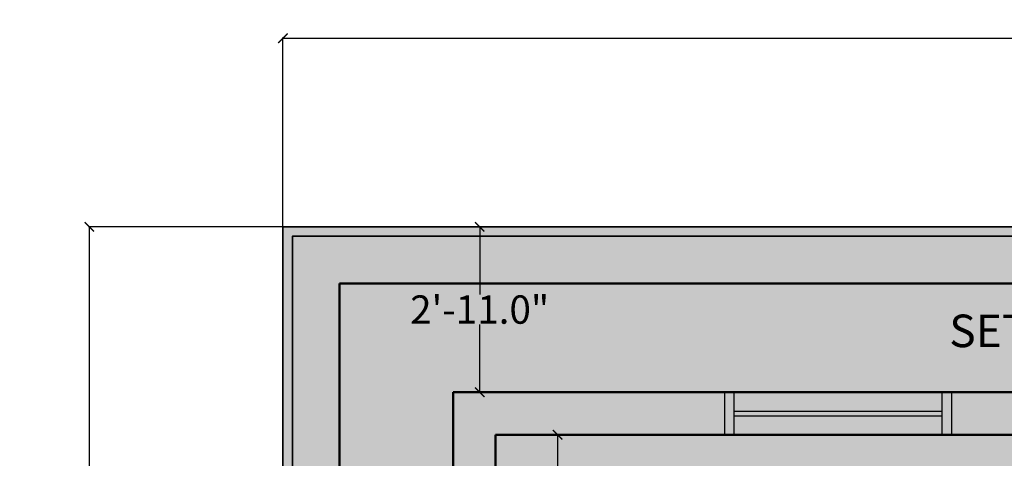
# Model space of a CAD drawing. Units: inches. Extents: x 528 to 2620, y -1066 to 798.
# Tile 9 of 41: x 528 to 737, y 705 to 798. Entities that reach past the tile are written whole.
import ezdxf

# ---------------------------------------------------------------- set-up
doc = ezdxf.new("R2010")
doc.units = ezdxf.units.IN
doc.header["$MEASUREMENT"] = 0
for name, color, linetype, lineweight in [('A-ANNO-DIMS', 2, 'Continuous', 18), ('A-AREA-IDEN', 7, 'Continuous', 18), ('A-GLAZ', 3, 'Continuous', 25), ('A-WALL', 7, 'Continuous', 50), ('A-WALL-PATT', 8, 'Continuous', 13), ('C-PROP', 5, 'Continuous', 35)]:
    doc.layers.add(name, color=color, linetype=linetype, lineweight=lineweight)
doc.styles.get("Standard").update_dxf_attribs({"font": 'arial.ttf'})
doc.dimstyles.get("Standard").update_dxf_attribs({"dimtxt": 6, "dimasz": 2, "dimexe": 0.18, "dimexo": 0.0625, "dimgap": 0.09, "dimtad": 0, "dimtih": 1, "dimtoh": 1, "dimdec": 1, "dimzin": 0, "dimdsep": 46, "dimlunit": 3, "dimtxsty": 'Standard', "dimblk": 'ARCHTICK', "dimcen": 0.09, "dimadec": 0, "dimazin": 0, "dimtfac": 1, "dimtdec": 1, "dimtofl": 0, "dimtmove": 0, "dimatfit": 3, "dimfxl": 1, "dimtolj": 1, "dimtzin": 0, "dimarcsym": 0})

# ---------------------------------------------------------------- blocks, each defined once
blk = doc.blocks.new('_ArchTick')
at = {"color": 0, "linetype": 'ByBlock', "const_width": 0.15}
blk.add_lwpolyline([(-0.5, -0.5), (0.5, 0.5)], dxfattribs=at)
blk = doc.blocks.new('*D11')
at = {"layer": 'A-ANNO-DIMS', "color": 0, "lineweight": -2, "transparency": 16777216}
for p, q in [((584.06, 753.98), (584.06, 794.01)), ((584.06, 793.83), (758.88, 793.83)), ((944.06, 793.83), (769.24, 793.83)), ((944.06, 753.98), (944.06, 794.01))]:
    blk.add_line(p, q, dxfattribs=at)
at = {"layer": 'Defpoints', "color": 0, "transparency": 16777216}
for p in [(944.06, 793.83), (584.06, 753.92), (944.06, 753.92)]:
    blk.add_point(p, dxfattribs=at)
at = {"layer": 'A-ANNO-DIMS', "color": 0, "lineweight": -2, "transparency": 16777216, "xscale": 2, "yscale": 2, "zscale": 2, "rotation": 180}
blk.add_blockref('_ArchTick', (584.06, 793.83), dxfattribs=at)
at = {"layer": 'A-ANNO-DIMS', "color": 0, "lineweight": -2, "transparency": 16777216, "xscale": 2, "yscale": 2, "zscale": 2}
blk.add_blockref('_ArchTick', (944.06, 793.83), dxfattribs=at)
at = {"layer": 'A-ANNO-DIMS', "color": 0, "transparency": 16777216, "insert": (764.06, 793.83), "char_height": 6, "attachment_point": 5}
blk.add_mtext("\\A1;30'", dxfattribs=at)
blk = doc.blocks.new('*D12')
at = {"layer": 'A-ANNO-DIMS', "color": 0, "lineweight": -2, "transparency": 16777216}
for p, q in [((584, 753.92), (542.88, 753.92)), ((543.06, 753.92), (543.06, 484.58)), ((543.06, 208.92), (543.06, 478.27)), ((584, 208.92), (542.88, 208.92))]:
    blk.add_line(p, q, dxfattribs=at)
at = {"layer": 'Defpoints', "color": 0, "transparency": 16777216}
for p in [(584.06, 753.92), (543.06, 208.92), (584.06, 208.92)]:
    blk.add_point(p, dxfattribs=at)
at = {"layer": 'A-ANNO-DIMS', "color": 0, "lineweight": -2, "transparency": 16777216, "xscale": 2, "yscale": 2, "zscale": 2}
for p, rotation in [((543.06, 753.92), 90), ((543.06, 208.92), 270)]:
    blk.add_blockref('_ArchTick', p, dxfattribs=dict(at, rotation=rotation))
at = {"layer": 'A-ANNO-DIMS', "color": 0, "transparency": 16777216, "insert": (543.06, 481.42), "char_height": 6, "attachment_point": 5}
blk.add_mtext('\\A1;45\'-5.0"', dxfattribs=at)
blk = doc.blocks.new('*D13')
at = {"layer": 'A-ANNO-DIMS', "color": 0, "lineweight": -2, "transparency": 16777216}
for p, q in [((625.99, 753.92), (625.52, 753.92)), ((625.7, 753.92), (625.7, 739.58)), ((625.7, 718.92), (625.7, 733.27)), ((625.99, 718.92), (625.52, 718.92))]:
    blk.add_line(p, q, dxfattribs=at)
at = {"layer": 'Defpoints', "color": 0, "transparency": 16777216}
for p in [(625.7, 753.92), (626.05, 753.92), (626.05, 718.92)]:
    blk.add_point(p, dxfattribs=at)
at = {"layer": 'A-ANNO-DIMS', "color": 0, "lineweight": -2, "transparency": 16777216, "xscale": 2, "yscale": 2, "zscale": 2}
for p, rotation in [((625.7, 753.92), 90), ((625.7, 718.92), 270)]:
    blk.add_blockref('_ArchTick', p, dxfattribs=dict(at, rotation=rotation))
at = {"layer": 'A-ANNO-DIMS', "color": 0, "transparency": 16777216, "insert": (625.7, 736.42), "char_height": 6, "attachment_point": 5}
blk.add_mtext('\\A1;2\'-11.0"', dxfattribs=at)
blk = doc.blocks.new('*D26')
at = {"layer": 'A-ANNO-DIMS', "color": 0, "lineweight": -2, "transparency": 16777216}
for p, q in [((642.51, 709.92), (641.99, 709.92)), ((642.17, 709.92), (642.17, 647.02)), ((642.17, 577.92), (642.17, 640.82)), ((642.51, 577.92), (641.99, 577.92))]:
    blk.add_line(p, q, dxfattribs=at)
at = {"layer": 'Defpoints', "color": 0, "transparency": 16777216}
for p in [(642.57, 709.92), (642.17, 577.92), (642.57, 577.92)]:
    blk.add_point(p, dxfattribs=at)
at = {"layer": 'A-ANNO-DIMS', "color": 0, "lineweight": -2, "transparency": 16777216, "xscale": 2, "yscale": 2, "zscale": 2}
for p, rotation in [((642.17, 709.92), 90), ((642.17, 577.92), 270)]:
    blk.add_blockref('_ArchTick', p, dxfattribs=dict(at, rotation=rotation))
at = {"layer": 'A-ANNO-DIMS', "color": 0, "transparency": 16777216, "insert": (642.17, 643.92), "char_height": 6, "attachment_point": 5}
blk.add_mtext("\\A1;11'", dxfattribs=at)
blk = doc.blocks.new('WIN-1200')
for p, q in [((677.56, 718.92), (725.56, 718.92)), ((677.56, 709.92), (677.56, 718.92)), ((679.56, 709.92), (679.56, 718.92)), ((723.56, 718.92), (723.56, 709.92)), ((725.56, 718.92), (725.56, 709.92)), ((679.56, 714.92), (723.56, 714.92)), ((679.56, 713.92), (723.56, 713.92)), ((725.56, 709.92), (677.56, 709.92))]:
    blk.add_line(p, q)

msp = doc.modelspace()

# ---------------------------------------------------------------- hatches: boundary and pattern name
at = {"layer": 'A-WALL-PATT', "transparency": 33554687}
h = msp.add_hatch(color=256, dxfattribs=at)
h.dxf.hatch_style = 1
h.paths.add_polyline_path([(944.06, 753.92), (584.06, 753.92), (584.06, 208.92), (608.06, 208.92), (608.06, 210.92), (586.06, 210.92), (586.06, 751.92), (942.06, 751.92), (942.06, 210.92), (728.06, 210.92), (728.06, 208.92), (944.06, 208.92)])
h = msp.add_hatch(color=256, dxfattribs=at)
h.dxf.hatch_style = 1
h.paths.add_polyline_path([(942.06, 751.92), (586.06, 751.92), (586.06, 210.92), (608.06, 210.92), (608.06, 220.92), (596.06, 220.92), (596.06, 741.92), (932.06, 741.92), (932.06, 220.92), (770.06, 220.92), (728.06, 220.92), (728.06, 210.92), (942.06, 210.92)])
at = {"layer": 'A-WALL-PATT', "transparency": 33554475}
h = msp.add_hatch(color=256, dxfattribs=at)
h.dxf.hatch_style = 1
h.paths.add_polyline_path([(620.06, 718.92), (908.06, 718.92), (908.06, 268.92), (770.06, 268.92), (770.06, 220.92), (932.06, 220.92), (932.06, 741.92), (596.06, 741.92), (596.06, 391.42), (620.06, 391.42)])
at = {"layer": 'A-WALL-PATT', "transparency": 33554687}
h = msp.add_hatch(color=256, dxfattribs=at)
h.dxf.hatch_style = 1
h.paths.add_polyline_path([(861.06, 273.92), (817.06, 273.92), (817.06, 272.92), (861.06, 272.92)])
h.paths.add_polyline_path([(817.06, 277.92), (815.06, 277.92), (815.06, 268.92), (817.06, 268.92)])
h.paths.add_polyline_path([(908.06, 397.92), (899.06, 397.92), (899.06, 395.92), (908.06, 395.92)])
h.paths.add_polyline_path([(908.06, 443.92), (899.06, 443.92), (899.06, 441.92), (908.06, 441.92)])
h.paths.add_polyline_path([(904.06, 441.92), (903.06, 441.92), (903.06, 397.92), (904.06, 397.92)])
h.paths.add_polyline_path([(625.06, 561.42), (624.06, 561.42), (624.06, 537.42), (625.06, 537.42)])
h.paths.add_polyline_path([(648.75, 334.44), (720.04, 334.44), (720.04, 345), (648.75, 345)], flags=9)
h.paths.add_polyline_path([(819.73, 323.15), (880.33, 323.15), (880.33, 333.71), (819.73, 333.71)], flags=9)
h.paths.add_polyline_path([(779.9, 680.61), (821.76, 680.61), (821.76, 691.17), (779.9, 691.17)], flags=9)
h.paths.add_polyline_path([(779.88, 692.36), (817.14, 692.36), (817.14, 703.06), (779.88, 703.06)], flags=9)
h.paths.add_polyline_path([(799.99, 453.88), (860.59, 453.88), (860.59, 464.44), (799.99, 464.44)], flags=9)
h.paths.add_polyline_path([(650.87, 539.4), (708.78, 539.4), (708.78, 549.95), (650.87, 549.95)], flags=9)
h.paths.add_polyline_path([(788.5, 612.01), (849.1, 612.01), (849.1, 622.56), (788.5, 622.56)], flags=9)
h.paths.add_polyline_path([(639.54, 648.31), (700.13, 648.31), (700.13, 658.87), (639.54, 658.87)], flags=9)
h.paths.add_polyline_path([(648.91, 346.09), (747.71, 346.09), (747.71, 356.78), (648.91, 356.78)], flags=9)
h.paths.add_polyline_path([(676.86, 450.66), (746.74, 450.66), (746.74, 461.36), (676.86, 461.36)], flags=9)
h.paths.add_polyline_path([(819.71, 334.95), (865.53, 334.95), (865.53, 345.64), (819.71, 345.64)], flags=9)
h.paths.add_polyline_path([(806.3, 467.75), (874.05, 467.75), (874.05, 478.44), (806.3, 478.44)], flags=9)
h.paths.add_polyline_path([(653.23, 552.28), (690.5, 552.28), (690.5, 562.98), (653.23, 562.98)], flags=9)
h.paths.add_polyline_path([(789.9, 623.41), (843.21, 623.41), (843.21, 634.1), (789.9, 634.1)], flags=9)
h.paths.add_polyline_path([(639.77, 662.1), (693.08, 662.1), (693.08, 672.8), (639.77, 672.8)], flags=9)
h.paths.add_polyline_path([(801.59, 242.91), (846.33, 242.91), (846.33, 253.6), (801.59, 253.6)], flags=9)
h.paths.add_polyline_path([(925.36, 593.98), (925.36, 674.06), (914.67, 674.06), (914.67, 593.98)], flags=9)
h.paths.add_polyline_path([(612.56, 593.98), (612.56, 674.06), (601.87, 674.06), (601.87, 593.98)], flags=9)
h.paths.add_polyline_path([(723.31, 726.56), (803.39, 726.56), (803.39, 737.25), (723.31, 737.25)], flags=9)
at = {"layer": 'A-WALL-PATT', "transparency": 33554521}
h = msp.add_hatch(color=256, dxfattribs=at)
h.dxf.hatch_style = 1
h.paths.add_polyline_path([(629.06, 709.92), (677.56, 709.92), (677.56, 718.92), (620.06, 718.92), (620.06, 667.92), (629.06, 667.92)])
h.paths.add_polyline_path([(790.56, 718.92), (725.56, 718.92), (725.56, 709.92), (774.06, 709.92), (774.06, 577.92), (768.48, 577.92), (768.56, 573.42), (774.06, 573.42), (774.06, 567.42), (778.56, 567.42), (778.56, 669.42), (831.06, 669.42), (831.06, 675.92), (826.56, 675.92), (826.56, 673.92), (778.56, 673.92), (778.56, 709.92), (790.56, 709.92)])
h.paths.add_polyline_path([(908.06, 718.92), (879.06, 718.92), (879.06, 709.92), (899.06, 709.92), (899.06, 641.67), (908.06, 641.67)])
h.paths.add_polyline_path([(629.06, 619.92), (620.06, 619.92), (620.06, 561.42), (629.06, 561.42), (629.06, 573.42), (724.06, 573.42), (724.06, 569.42), (728.56, 569.42), (728.56, 577.92), (629.06, 577.92)])
h.paths.add_polyline_path([(779.06, 391.42), (779.06, 400.42), (770.06, 400.42), (764.06, 400.42), (764.06, 397.42), (764.06, 391.42), (770.06, 391.42), (770.06, 268.92), (815.06, 268.92), (815.06, 277.92), (779.06, 277.92), (779.06, 359.77)])
h.paths.add_polyline_path([(908.06, 395.92), (899.06, 395.92), (851.06, 395.92), (851.06, 391.42), (899.06, 391.42), (899.06, 277.92), (863.06, 277.92), (863.06, 268.92), (908.06, 268.92)])
h.paths.add_polyline_path([(908.06, 593.67), (899.06, 593.67), (899.06, 525.42), (778.56, 525.42), (778.56, 527.17), (774.06, 527.17), (774.06, 520.92), (899.06, 520.92), (899.06, 443.92), (908.06, 443.92)])
h.paths.add_polyline_path([(629.06, 520.92), (728.56, 520.92), (728.56, 545.42), (724.06, 545.42), (724.06, 525.42), (629.06, 525.42), (629.06, 537.42), (620.06, 537.42), (620.06, 484.67), (629.06, 484.67)])
h.paths.add_polyline_path([(629.06, 436.67), (620.06, 436.67), (620.06, 391.42), (648.56, 391.42), (648.56, 400.42), (629.06, 400.42)])
h.paths.add_polyline_path([(716.06, 397.42), (716.06, 400.42), (696.56, 400.42), (696.56, 391.42), (716.06, 391.42)])
at = {"layer": 'A-WALL-PATT', "transparency": 33554681}
h = msp.add_hatch(color=256, dxfattribs=at)
h.dxf.hatch_style = 1
h.paths.add_polyline_path([(629.06, 665.92), (625.06, 665.92), (625.06, 621.92), (629.06, 621.92)])
h.paths.add_polyline_path([(624.06, 665.92), (620.06, 665.92), (620.06, 621.92), (624.06, 621.92)])
h.paths.add_polyline_path([(723.56, 713.92), (679.56, 713.92), (679.56, 709.92), (723.56, 709.92)])
h.paths.add_polyline_path([(723.56, 718.92), (679.56, 718.92), (679.56, 714.92), (723.56, 714.92)])
h.paths.add_polyline_path([(814.56, 713.92), (790.56, 713.92), (790.56, 709.92), (814.56, 709.92)])
h.paths.add_polyline_path([(814.56, 718.92), (790.56, 718.92), (790.56, 714.92), (814.56, 714.92)])
h.paths.add_polyline_path([(877.06, 713.92), (833.06, 713.92), (833.06, 709.92), (877.06, 709.92)])
h.paths.add_polyline_path([(877.06, 718.92), (833.06, 718.92), (833.06, 714.92), (877.06, 714.92)])
h.paths.add_polyline_path([(908.06, 639.67), (904.06, 639.67), (904.06, 595.67), (908.06, 595.67)])
h.paths.add_polyline_path([(903.06, 639.67), (899.06, 639.67), (899.06, 595.67), (903.06, 595.67)])
h.paths.add_polyline_path([(908.06, 441.92), (904.06, 441.92), (904.06, 397.92), (908.06, 397.92)])
h.paths.add_polyline_path([(903.06, 441.92), (899.06, 441.92), (899.06, 397.92), (903.06, 397.92)])
h.paths.add_polyline_path([(861.06, 272.92), (817.06, 272.92), (817.06, 268.92), (861.06, 268.92)])
h.paths.add_polyline_path([(861.06, 277.92), (817.06, 277.92), (817.06, 273.92), (861.06, 273.92)])
h.paths.add_polyline_path([(694.56, 395.42), (650.56, 395.42), (650.56, 391.42), (694.56, 391.42)])
h.paths.add_polyline_path([(694.56, 400.42), (650.56, 400.42), (650.56, 396.42), (694.56, 396.42)])
h.paths.add_polyline_path([(629.06, 482.67), (625.06, 482.67), (625.06, 438.67), (629.06, 438.67)])
h.paths.add_polyline_path([(624.06, 482.67), (620.06, 482.67), (620.06, 438.67), (624.06, 438.67)])
h.paths.add_polyline_path([(629.06, 561.42), (625.06, 561.42), (625.06, 537.42), (629.06, 537.42)])
h.paths.add_polyline_path([(624.06, 561.42), (620.06, 561.42), (620.06, 537.42), (624.06, 537.42)])
h = msp.add_hatch(color=256, dxfattribs=at)
h.dxf.hatch_style = 1
h.paths.add_polyline_path([(625.06, 665.92), (624.06, 665.92), (624.06, 621.92), (625.06, 621.92)])
h.paths.add_polyline_path([(629.06, 667.92), (620.06, 667.92), (620.06, 665.92), (629.06, 665.92)])
h.paths.add_polyline_path([(629.06, 621.92), (620.06, 621.92), (620.06, 619.92), (629.06, 619.92)])
h.paths.add_polyline_path([(723.56, 714.92), (679.56, 714.92), (679.56, 713.92), (723.56, 713.92)])
h.paths.add_polyline_path([(725.56, 718.92), (723.56, 718.92), (723.56, 709.92), (725.56, 709.92)])
h.paths.add_polyline_path([(679.56, 718.92), (677.56, 718.92), (677.56, 709.92), (679.56, 709.92)])
h.paths.add_polyline_path([(814.56, 714.92), (790.56, 714.92), (790.56, 713.92), (814.56, 713.92)])
h.paths.add_polyline_path([(877.06, 714.92), (833.06, 714.92), (833.06, 713.92), (877.06, 713.92)])
h.paths.add_polyline_path([(879.06, 718.92), (877.06, 718.92), (877.06, 709.92), (879.06, 709.92)])
h.paths.add_polyline_path([(833.06, 718.92), (831.06, 718.92), (831.06, 709.92), (833.06, 709.92)])
h.paths.add_polyline_path([(650.56, 400.42), (648.56, 400.42), (648.56, 391.42), (650.56, 391.42)])
h.paths.add_polyline_path([(694.56, 396.42), (650.56, 396.42), (650.56, 395.42), (694.56, 395.42)])
h.paths.add_polyline_path([(696.56, 400.42), (694.56, 400.42), (694.56, 391.42), (696.56, 391.42)])
h.paths.add_polyline_path([(629.06, 438.67), (620.06, 438.67), (620.06, 436.67), (629.06, 436.67)])
h.paths.add_polyline_path([(629.06, 484.67), (620.06, 484.67), (620.06, 482.67), (629.06, 482.67)])
h.paths.add_polyline_path([(625.06, 482.67), (624.06, 482.67), (624.06, 438.67), (625.06, 438.67)])
at = {"layer": 'A-WALL-PATT', "transparency": 33554590}
h = msp.add_hatch(color=256, dxfattribs=at)
h.dxf.hatch_style = 1
h.paths.add_polyline_path([(774.06, 709.92), (629.06, 709.92), (629.06, 577.92), (728.56, 577.92), (728.56, 579.42), (728.56, 619.42), (730.31, 619.42), (730.31, 619.38, -0.401453), (768.56, 579.42), (768.56, 577.92), (774.06, 577.92)])
h.paths.add_polyline_path([(723.9, 686.06), (723.97, 686.06), (723.83, 686.13)], flags=0)
h.paths.add_polyline_path([(722.79, 642.7), (722.89, 642.76), (722.89, 684.99), (722.65, 685.24), (722.65, 685.82), (723.08, 686.26), (723.53, 686.26), (723.97, 686.06), (724.74, 686.13), (770.7, 686.13), (770.78, 686.14), (771.13, 686.27), (771.69, 686.09), (771.94, 685.48), (771.67, 684.9), (771.58, 684.87), (771.58, 642.78), (771.88, 642.51), (771.88, 641.92), (771.51, 641.46), (770.85, 641.46), (770.4, 641.83), (770.4, 641.55), (724.74, 641.55), (723.99, 641.7), (723.44, 641.41), (722.88, 641.59), (722.6, 642.14)], flags=16)
h.paths.add_polyline_path([(723.99, 641.7), (723.99, 641.71), (723.99, 641.7)], flags=0)
h.paths.add_polyline_path([(722.89, 642.73), (722.89, 684.99), (722.65, 685.24), (722.65, 685.82), (723.08, 686.26), (723.29, 686.26), (722.99, 686.17), (722.79, 685.97), (722.65, 685.68), (722.65, 685.43), (722.75, 685.14), (722.94, 684.94), (723.24, 684.81), (723.48, 684.81), (723.78, 684.9), (723.98, 685.1), (724.17, 685.49), (724.12, 685.64), (724.12, 685.25), (723.63, 684.75), (723.63, 642.96), (724.12, 642.51), (724.12, 641.89), (723.66, 641.46), (723.08, 641.46), (722.65, 641.9), (722.65, 642.48)], flags=0)
h.paths.add_polyline_path([(722.65, 642.29), (722.65, 642.04), (722.79, 641.75), (723.08, 641.46), (723.29, 641.46), (722.88, 641.59), (722.6, 642.14)], flags=0)
h.paths.add_polyline_path([(770.75, 686.13), (770.58, 686.13), (770.55, 686.06)], flags=0)
h.paths.add_polyline_path([(743.3, 645.29), (753.23, 659.4), (748.69, 663.75), (753.23, 668.54), (743.3, 682.46), (743.79, 682.59), (744.14, 682.68), (744.53, 682.93), (744.63, 683.08), (745.02, 683.33), (744.53, 684.07), (744.78, 684.16), (744.87, 684.31), (745.51, 684.4), (746.08, 684.65), (746.47, 684.65), (746.82, 684.81), (747.46, 685.03), (747.71, 685.14), (748.2, 685.28), (748.39, 685.52), (748.86, 685.52), (749.99, 686.13), (753.49, 676.03), (757.38, 680.15), (757.79, 679.76), (758.04, 680.65), (758.29, 681.23), (758.29, 682.05), (758.02, 682.59), (757.87, 683.17), (757.82, 683.78), (758.39, 684.07), (758.98, 684.2), (759.62, 684.16), (760.21, 683.96), (760.75, 683.67), (761.86, 683.67), (762.4, 683.96), (762.99, 684.11), (763.63, 684.11), (764.2, 683.96), (764.74, 683.67), (766.12, 683.67), (766.66, 683.96), (767.25, 684.16), (767.87, 684.2), (768.46, 684.07), (769.05, 683.78), (769, 683.17), (768.85, 682.59), (768.55, 682.05), (768.55, 681.23), (768.8, 680.65), (769.09, 679.75), (768.95, 678.83), (768.8, 678.23), (768.55, 677.65), (768.55, 676.82), (768.8, 676.24), (769.09, 675.34), (768.95, 674.42), (768.8, 673.82), (768.55, 673.28), (768.55, 672.41), (768.8, 671.87), (769, 671.29), (769.05, 670.64), (768.95, 670.02), (768.8, 669.41), (768.55, 668.87), (768.55, 668), (768.97, 667.24), (769.05, 666.28), (769.05, 665.56), (768.46, 665.32), (767.87, 665.16), (767.25, 665.16), (766.66, 665.36), (766.12, 665.7), (764.74, 665.7), (763.94, 665.2), (762.99, 665.2), (762.4, 665.36), (761.86, 665.7), (761, 665.7), (762.7, 664.09), (760.74, 662.03), (761.86, 662.03), (762.4, 662.32), (763.34, 662.55), (764.25, 662.32), (764.79, 662.03), (766.12, 662.03), (766.66, 662.32), (767.25, 662.52), (767.87, 662.56), (768.51, 662.43), (769.05, 662.12), (769.05, 661.4), (769.05, 660.8), (768.85, 660.21), (768.55, 659.68), (768.55, 658.85), (768.85, 658.27), (769, 657.66), (769.07, 656.75), (768.85, 655.85), (768.55, 655.27), (768.55, 654.44), (768.85, 653.86), (769.07, 652.96), (769, 652.05), (768.85, 651.44), (768.55, 650.91), (768.55, 650.03), (768.85, 649.5), (769, 648.91), (769.05, 648.26), (769, 647.64), (768.85, 647.03), (768.55, 646.5), (768.55, 645.62), (768.85, 645.09), (769.05, 644.55), (769.05, 643.9), (768.51, 643.65), (767.87, 643.52), (767.25, 643.52), (766.66, 643.72), (766.12, 644.06), (764.79, 644.06), (764.25, 643.72), (763.34, 643.49), (762.4, 643.72), (761.86, 644.06), (760.8, 644.06), (760.26, 643.72), (759.67, 643.52), (759.03, 643.52), (758.39, 643.65), (757.87, 643.9), (757.87, 644.55), (758.04, 645.09), (758.34, 645.62), (758.34, 646.5), (758.04, 647.03), (757.92, 647.64), (757.87, 648.06), (757.38, 647.59), (753.42, 651.77), (749.99, 641.62), (749.5, 641.71), (749.35, 641.95), (748.54, 642.45), (747.31, 642.94), (746.65, 642.94), (746.33, 643.18), (745.51, 643.57), (744.53, 643.65), (745.01, 644.4), (744.63, 644.64), (744.14, 644.89), (743.79, 645.13)], flags=0)
h.paths.add_polyline_path([(755.66, 654.93), (756.54, 654.69), (757.53, 654.33), (756.64, 654.58)], flags=0)
h.paths.add_polyline_path([(758.34, 649.2), (758.34, 648.71), (758.59, 644.3), (758.59, 648.8)], flags=0)
h.paths.add_polyline_path([(758.34, 649.29), (758.09, 649.7), (758.36, 649.17)], flags=0)
h.paths.add_polyline_path([(755.66, 672.79), (756.49, 673.04), (757.36, 673.35), (757.35, 673.36), (756.64, 673.15)], flags=0)
h.paths.add_polyline_path([(760.26, 639.64), (771.41, 639.64), (771.41, 624.04), (760.26, 624.04)], flags=16)
h.paths.add_polyline_path([(761.38, 638.53), (770.29, 638.53), (770.29, 625.15), (761.38, 625.15)], flags=0)
edge = h.paths.add_edge_path(flags=0)
edge.add_ellipse((765.84, 631.84), major_axis=(-2.24, 2.24), ratio=1, start_angle=-45, end_angle=45, ccw=False)
edge.add_ellipse((765.84, 631.84), major_axis=(-2.24, 2.24), ratio=1, start_angle=-135, end_angle=-45, ccw=False)
edge.add_ellipse((765.84, 631.84), major_axis=(-2.24, 2.24), ratio=1, start_angle=135, end_angle=-135, ccw=False)
edge.add_ellipse((765.84, 631.84), major_axis=(-2.24, 2.24), ratio=1, start_angle=45, end_angle=135, ccw=False)
h.paths.add_polyline_path([(758.59, 683.42), (758.59, 678.92), (758.37, 678.58), (758.34, 678.43), (758.09, 678.05), (758.34, 678.52), (758.34, 679.01)], flags=0)
h.paths.add_polyline_path([(760.26, 688.04), (760.26, 703.64), (771.41, 703.64), (771.41, 688.04)], flags=16)
h.paths.add_polyline_path([(770.4, 685.39), (770.4, 685.85), (770.85, 686.22), (771.51, 686.22), (771.88, 685.76), (771.88, 685.17), (771.58, 684.9), (771.58, 642.78), (771.88, 642.51), (771.88, 641.92), (771.51, 641.46), (770.85, 641.46), (770.4, 641.83), (770.4, 642.29)], flags=0)
h.paths.add_polyline_path([(770.53, 642.68), (771.05, 643.01), (771.67, 642.77), (771.94, 642.2), (771.69, 641.59), (771.13, 641.41), (770.55, 641.62), (770.35, 642.13)], flags=16)
h.paths.add_polyline_path([(761.38, 689.15), (761.38, 702.53), (770.29, 702.53), (770.29, 689.15)], flags=0)
edge = h.paths.add_edge_path(flags=0)
edge.add_ellipse((765.84, 695.84), major_axis=(2.24, 2.24), ratio=1, start_angle=405, end_angle=495, ccw=False)
edge.add_ellipse((765.84, 695.84), major_axis=(2.24, 2.24), ratio=1, start_angle=675, end_angle=765, ccw=False)
edge.add_ellipse((765.84, 695.84), major_axis=(2.24, 2.24), ratio=1, start_angle=585, end_angle=675, ccw=False)
edge.add_ellipse((765.84, 695.84), major_axis=(2.24, 2.24), ratio=1, start_angle=495, end_angle=585, ccw=False)
h.paths.add_polyline_path([(770.7, 684.9), (770.94, 684.74), (771.41, 684.74), (771.73, 685.03), (771.88, 685.34), (771.88, 685.64), (771.69, 686.09), (771.58, 686.13), (771.88, 685.76), (771.88, 685.17), (771.41, 684.74), (770.85, 684.74)], flags=0)
h.paths.add_polyline_path([(899.06, 709.92), (831.06, 709.92), (831.06, 699.92), (829.81, 699.92), (829.81, 675.92), (831.06, 675.92), (831.06, 669.42), (778.56, 669.42), (778.56, 567.17), (780.06, 567.17), (820.06, 567.17), (820.06, 565.42), (820.02, 565.42, -0.401453), (780.06, 527.17), (778.56, 527.17), (778.56, 525.42), (899.06, 525.42)])
h.paths.add_polyline_path([(849.2, 636.01), (849.27, 636.02), (849.13, 636.08)], flags=0)
h.paths.add_polyline_path([(848.19, 634.95), (847.95, 635.2), (847.95, 635.78), (848.38, 636.22), (848.83, 636.22), (849.27, 636.02), (850.04, 636.08), (896, 636.08), (896.08, 636.1), (896.43, 636.22), (896.99, 636.05), (897.24, 635.43), (896.97, 634.86), (896.88, 634.83), (896.88, 592.74), (897.18, 592.47), (897.18, 591.88), (896.81, 591.42), (896.15, 591.42), (895.7, 591.79), (895.7, 591.51), (850.04, 591.51), (849.29, 591.66), (848.74, 591.37), (848.18, 591.54), (847.9, 592.1), (848.09, 592.65), (848.19, 592.71)], flags=16)
h.paths.add_polyline_path([(849.29, 591.66), (849.29, 591.66), (849.29, 591.66)], flags=16)
h.paths.add_polyline_path([(848.19, 634.95), (847.95, 635.2), (847.95, 635.78), (848.38, 636.22), (848.59, 636.22), (848.29, 636.13), (848.09, 635.93), (847.95, 635.64), (847.95, 635.39), (848.05, 635.1), (848.24, 634.9), (848.54, 634.76), (848.78, 634.76), (849.08, 634.85), (849.28, 635.05), (849.47, 635.44), (849.42, 635.59), (849.42, 635.21), (848.93, 634.7), (848.93, 592.92), (849.42, 592.47), (849.42, 591.84), (848.96, 591.42), (848.38, 591.42), (847.95, 591.86), (847.95, 592.44), (848.19, 592.69)], flags=0)
h.paths.add_polyline_path([(847.95, 592.25), (847.95, 592), (848.09, 591.71), (848.38, 591.42), (848.59, 591.42), (848.18, 591.54), (847.9, 592.1)], flags=16)
h.paths.add_polyline_path([(896.05, 636.08), (895.88, 636.08), (895.85, 636.01)], flags=0)
h.paths.add_polyline_path([(868.6, 632.41), (869.09, 632.55), (869.44, 632.64), (869.83, 632.88), (869.93, 633.04), (870.32, 633.28), (869.83, 634.02), (870.08, 634.11), (870.17, 634.27), (870.81, 634.36), (871.38, 634.61), (871.77, 634.61), (872.12, 634.76), (872.76, 634.99), (873.01, 635.1), (873.5, 635.23), (873.69, 635.48), (874.16, 635.48), (875.29, 636.08), (878.79, 625.99), (882.68, 630.11), (883.09, 629.71), (883.34, 630.6), (883.59, 631.18), (883.59, 632.01), (883.32, 632.55), (883.17, 633.13), (883.12, 633.73), (883.69, 634.02), (884.28, 634.16), (884.92, 634.11), (885.51, 633.91), (886.05, 633.62), (887.16, 633.62), (887.7, 633.91), (888.29, 634.07), (888.93, 634.07), (889.5, 633.91), (890.04, 633.62), (891.42, 633.62), (891.96, 633.91), (892.55, 634.11), (893.17, 634.16), (893.76, 634.02), (894.35, 633.73), (894.3, 633.13), (894.15, 632.55), (893.85, 632.01), (893.85, 631.18), (894.1, 630.6), (894.39, 629.71), (894.25, 628.79), (894.1, 628.18), (893.85, 627.6), (893.85, 626.77), (894.1, 626.19), (894.39, 625.3), (894.25, 624.38), (894.1, 623.78), (893.85, 623.24), (893.85, 622.37), (894.1, 621.83), (894.3, 621.25), (894.35, 620.6), (894.25, 619.97), (894.1, 619.37), (893.85, 618.83), (893.85, 617.96), (894.27, 617.2), (894.35, 616.23), (894.35, 615.52), (893.76, 615.27), (893.17, 615.12), (892.55, 615.12), (891.96, 615.32), (891.42, 615.65), (890.04, 615.65), (889.25, 615.16), (888.29, 615.16), (887.7, 615.32), (887.16, 615.65), (886.31, 615.65), (888, 614.04), (886.04, 611.98), (887.16, 611.98), (887.7, 612.27), (888.64, 612.5), (889.55, 612.27), (890.09, 611.98), (891.42, 611.98), (891.96, 612.27), (892.55, 612.48), (893.17, 612.52), (893.81, 612.39), (894.35, 612.07), (894.35, 611.36), (894.35, 610.75), (894.15, 610.17), (893.85, 609.63), (893.85, 608.81), (894.15, 608.22), (894.3, 607.62), (894.37, 606.7), (894.15, 605.81), (893.85, 605.22), (893.85, 604.4), (894.15, 603.81), (894.37, 602.92), (894.3, 602), (894.15, 601.4), (893.85, 600.86), (893.85, 599.99), (894.15, 599.45), (894.3, 598.87), (894.35, 598.22), (894.3, 597.59), (894.15, 596.99), (893.85, 596.45), (893.85, 595.58), (894.15, 595.04), (894.35, 594.51), (894.35, 593.86), (893.81, 593.61), (893.17, 593.48), (892.55, 593.48), (891.96, 593.68), (891.42, 594.01), (890.09, 594.01), (889.55, 593.68), (888.64, 593.45), (887.7, 593.68), (887.16, 594.01), (886.1, 594.01), (885.56, 593.68), (884.97, 593.48), (884.33, 593.48), (883.69, 593.61), (883.17, 593.86), (883.17, 594.51), (883.34, 595.04), (883.64, 595.58), (883.64, 596.45), (883.34, 596.99), (883.22, 597.59), (883.17, 598.01), (882.68, 597.55), (878.72, 601.73), (875.29, 591.57), (874.8, 591.66), (874.65, 591.91), (873.84, 592.4), (872.61, 592.89), (871.95, 592.89), (871.63, 593.14), (870.81, 593.52), (869.83, 593.61), (870.31, 594.36), (869.93, 594.6), (869.44, 594.84), (869.09, 595.09), (868.6, 595.24), (878.53, 609.35), (873.99, 613.71), (878.53, 618.49)], flags=0)
h.paths.add_polyline_path([(880.96, 622.75), (881.79, 622.99), (882.66, 623.31), (882.65, 623.31), (881.94, 623.1)], flags=0)
h.paths.add_polyline_path([(880.96, 604.89), (881.84, 604.64), (882.83, 604.28), (881.94, 604.53)], flags=16)
h.paths.add_polyline_path([(883.39, 628.01), (883.64, 628.48), (883.64, 628.97), (883.89, 633.38), (883.89, 628.88), (883.67, 628.53), (883.64, 628.39)], flags=0)
h.paths.add_polyline_path([(883.64, 599.16), (883.64, 598.67), (883.89, 594.26), (883.89, 598.76)], flags=16)
h.paths.add_polyline_path([(883.64, 599.25), (883.39, 599.65), (883.66, 599.12)], flags=16)
h.paths.add_polyline_path([(885.56, 637.99), (885.56, 653.6), (896.71, 653.6), (896.71, 637.99)], flags=16)
h.paths.add_polyline_path([(885.56, 589.6), (896.71, 589.6), (896.71, 573.99), (885.56, 573.99)], flags=16)
h.paths.add_polyline_path([(886.68, 639.11), (886.68, 652.48), (895.59, 652.48), (895.59, 639.11)], flags=0)
h.paths.add_polyline_path([(886.68, 588.48), (895.59, 588.48), (895.59, 575.11), (886.68, 575.11)], flags=0)
edge = h.paths.add_edge_path(flags=0)
edge.add_ellipse((891.14, 645.79), major_axis=(2.24, 2.24), ratio=1, start_angle=405, end_angle=495, ccw=False)
edge.add_ellipse((891.14, 645.79), major_axis=(2.24, 2.24), ratio=1, start_angle=675, end_angle=765, ccw=False)
edge.add_ellipse((891.14, 645.79), major_axis=(2.24, 2.24), ratio=1, start_angle=585, end_angle=675, ccw=False)
edge.add_ellipse((891.14, 645.79), major_axis=(2.24, 2.24), ratio=1, start_angle=495, end_angle=585, ccw=False)
edge = h.paths.add_edge_path(flags=0)
edge.add_ellipse((891.14, 581.8), major_axis=(-2.24, 2.24), ratio=1, start_angle=-45, end_angle=45, ccw=False)
edge.add_ellipse((891.14, 581.8), major_axis=(-2.24, 2.24), ratio=1, start_angle=-135, end_angle=-45, ccw=False)
edge.add_ellipse((891.14, 581.8), major_axis=(-2.24, 2.24), ratio=1, start_angle=135, end_angle=-135, ccw=False)
edge.add_ellipse((891.14, 581.8), major_axis=(-2.24, 2.24), ratio=1, start_angle=45, end_angle=135, ccw=False)
h.paths.add_polyline_path([(895.7, 635.35), (895.7, 635.8), (896.15, 636.17), (896.81, 636.17), (897.18, 635.71), (897.18, 635.12), (896.88, 634.85), (896.88, 592.74), (897.18, 592.47), (897.18, 591.88), (896.81, 591.42), (896.15, 591.42), (895.7, 591.79), (895.7, 592.25)], flags=0)
h.paths.add_polyline_path([(896, 634.85), (896.24, 634.7), (896.71, 634.7), (897.03, 634.99), (897.18, 635.3), (897.18, 635.59), (896.99, 636.05), (896.88, 636.08), (897.18, 635.71), (897.18, 635.12), (896.71, 634.7), (896.15, 634.7)], flags=0)
h.paths.add_polyline_path([(895.83, 592.63), (896.35, 592.96), (896.97, 592.73), (897.24, 592.16), (896.99, 591.54), (896.43, 591.37), (895.85, 591.58), (895.65, 592.09)], flags=16)
h.paths.add_polyline_path([(725.25, 569.42), (724.06, 569.42), (724.06, 573.42), (629.06, 573.42), (629.06, 525.42), (724.06, 525.42), (724.06, 545.42), (725.25, 545.42)])
h.paths.add_polyline_path([(820.02, 565.42), (780.06, 565.42), (780.06, 567.17), (774.06, 567.17), (774.06, 567.42), (774.06, 573.42), (768.56, 573.42), (768.48, 577.92), (768.56, 577.92), (768.56, 579.42, 0.401453), (730.31, 619.38), (730.31, 579.42), (728.56, 579.42), (728.56, 573.42), (728.56, 569.42), (727.25, 569.42), (727.25, 545.42), (728.56, 545.42), (728.56, 520.92), (665.06, 520.92), (665.06, 436.42), (716.06, 436.42), (716.06, 421.42), (717.81, 421.42), (717.81, 421.36, -0.392996), (740.06, 397.42, -0.392996), (762.31, 421.36), (762.31, 421.42), (764.06, 421.42), (764.06, 400.42), (770.06, 400.42), (779.06, 400.42), (779.06, 391.42), (779.06, 359.77), (795.43, 359.77), (795.43, 294.3), (893.67, 294.3), (893.67, 277.92), (899.06, 277.92), (899.06, 391.42), (851.06, 391.42), (851.06, 395.92), (899.06, 395.92), (899.06, 443.92), (899.06, 520.92), (774.06, 520.92), (774.06, 527.17), (778.56, 527.17), (780.06, 527.17, 0.401453)])
h.paths.add_polyline_path([(774.06, 519.66), (842.12, 519.66), (842.12, 505.07), (788.64, 505.07), (788.64, 474.08), (788.64, 470.43, -0.883215), (779.53, 456.66), (774.97, 456.66, -0.414214), (774.06, 457.57)], flags=16)
h.paths.add_polyline_path([(775.88, 517.83), (840.3, 517.83), (840.3, 514.19), (788.64, 514.19), (788.64, 484.41), (779.53, 484.41), (779.53, 474.08), (775.88, 474.08)], flags=0)
h.paths.add_polyline_path([(706.7, 501.56, -0.254069), (706.7, 493.02), (698.31, 492.55), (698.31, 502.03)], flags=16)
h.paths.add_polyline_path([(691.33, 515.69), (691.8, 507.3), (682.32, 507.3), (682.79, 515.69, -0.254069)], flags=16)
h.paths.add_polyline_path([(695.49, 504.68), (695.49, 479.42), (678.64, 479.42), (678.64, 504.68)], flags=16)
h.paths.add_polyline_path([(706.7, 489.6, -0.254069), (706.7, 481.06), (698.31, 480.59), (698.31, 490.07)], flags=16)
h.paths.add_polyline_path([(675.81, 502.03), (675.81, 492.55), (667.42, 493.02, -0.254069), (667.42, 501.56)], flags=16)
h.paths.add_polyline_path([(691.8, 476.8), (691.33, 468.41, -0.254069), (682.79, 468.41), (682.32, 476.8)], flags=16)
h.paths.add_polyline_path([(675.81, 490.07), (675.81, 480.59), (667.42, 481.06, -0.254069), (667.42, 489.6)], flags=16)
h.paths.add_polyline_path([(764.06, 397.42), (762.31, 397.42), (762.31, 421.36, 0.392996), (740.06, 397.42, 0.392996), (717.81, 421.36), (717.81, 397.42), (716.06, 397.42), (716.06, 391.42), (716.06, 385.42), (764.06, 385.42), (764.06, 391.42)], flags=17)
h.paths.add_polyline_path([(716.06, 436.42), (705.86, 436.42), (705.86, 418.42), (716.06, 418.42), (716.06, 421.42)], flags=17)
h.paths.add_polyline_path([(716.06, 418.42), (705.86, 418.42), (705.86, 400.42), (716.06, 400.42)], flags=17)
h.paths.add_polyline_path([(705.86, 418.42), (695.66, 418.42), (695.66, 400.42), (696.56, 400.42), (705.86, 400.42)], flags=17)
h.paths.add_polyline_path([(705.86, 436.42), (695.66, 436.42), (695.66, 418.42), (705.86, 418.42)], flags=17)
h.paths.add_polyline_path([(695.66, 418.42), (685.46, 418.42), (685.46, 400.42), (695.66, 400.42)], flags=17)
h.paths.add_polyline_path([(695.66, 436.42), (685.46, 436.42), (685.46, 418.42), (695.66, 418.42)], flags=17)
h.paths.add_polyline_path([(685.46, 418.42), (675.26, 418.42), (675.26, 400.42), (685.46, 400.42)], flags=17)
h.paths.add_polyline_path([(685.46, 436.42), (675.26, 436.42), (675.26, 418.42), (685.46, 418.42)], flags=17)
h.paths.add_polyline_path([(675.26, 436.42), (665.06, 436.42), (665.06, 418.42), (675.26, 418.42)])
h.paths.add_polyline_path([(675.26, 418.42), (665.06, 418.42), (665.06, 400.42), (675.26, 400.42)])
h.paths.add_polyline_path([(665.06, 418.42), (646.97, 418.42), (646.99, 436.42), (629.06, 436.42), (629.06, 400.42), (665.06, 400.42)])
h.paths.add_polyline_path([(665.06, 436.42), (646.99, 436.42), (646.97, 418.42), (665.06, 418.42)], flags=17)
h.paths.add_polyline_path([(647.01, 446.62), (629.06, 446.62), (629.06, 436.67), (629.06, 436.42), (646.99, 436.42)])
h.paths.add_polyline_path([(665.06, 446.62), (647.01, 446.62), (646.99, 436.42), (665.06, 436.42)])
h.paths.add_polyline_path([(647.02, 456.82), (629.06, 456.82), (629.06, 446.62), (647.01, 446.62)])
h.paths.add_polyline_path([(665.06, 456.82), (647.02, 456.82), (647.01, 446.62), (665.06, 446.62)])
h.paths.add_polyline_path([(647.03, 467.02), (629.06, 467.02), (629.06, 456.82), (647.02, 456.82)])
h.paths.add_polyline_path([(665.06, 467.02), (647.03, 467.02), (647.02, 456.82), (665.06, 456.82)])
h.paths.add_polyline_path([(665.06, 477.22), (647.05, 477.22), (647.03, 467.02), (665.06, 467.02)])
h.paths.add_polyline_path([(647.05, 477.22), (629.06, 477.22), (629.06, 467.02), (647.03, 467.02)])
h.paths.add_polyline_path([(647.06, 487.22), (629.06, 487.22), (629.06, 477.22), (647.05, 477.22), (647.05, 479.02), (645.53, 483.25), (640.88, 480.37)])
h.paths.add_polyline_path([(665.06, 520.92), (629.06, 520.92), (629.06, 487.22), (647.06, 487.22), (665.06, 487.22)])
h.paths.add_polyline_path([(665.06, 487.22), (647.06, 487.22), (653.22, 480.35), (648.58, 483.24), (647.05, 479.02), (647.05, 477.22), (665.06, 477.22)])

# ---------------------------------------------------------------- linework, layer by layer
at = {"layer": 'A-WALL'}
for p, q in [((932.06, 741.92), (596.06, 741.92)), ((596.06, 741.92), (596.06, 391.42)), ((908.06, 718.92), (620.06, 718.92)), ((620.06, 718.92), (620.06, 391.42)), ((629.06, 709.92), (629.06, 577.92)), ((774.06, 709.92), (629.06, 709.92))]:
    msp.add_line(p, q, dxfattribs=at)
at = {"layer": 'C-PROP'}
for points in [[(728.06, 208.92), (944.06, 208.92), (944.06, 753.92), (584.06, 753.92), (584.06, 208.92), (608.06, 208.92)], [(728.06, 210.92), (942.06, 210.92), (942.06, 751.92), (586.06, 751.92), (586.06, 210.92), (608.06, 210.92)]]:
    msp.add_lwpolyline(points, dxfattribs=at)
msp.add_lwpolyline([(596.06, 741.92), (596.06, 220.92), (932.06, 220.92), (932.06, 741.92)], close=True, dxfattribs=at)

# ---------------------------------------------------------------- block references
at = {"layer": 'A-GLAZ'}
msp.add_blockref('WIN-1200', (0, 0), dxfattribs=at)

# ---------------------------------------------------------------- texts
at = {"layer": 'A-AREA-IDEN'}
msp.add_text('SET BACK AREA', height=6.8907, dxfattribs=at).set_placement((725.09, 728.46))

# ---------------------------------------------------------------- dimensions: what is measured, and where the dimension line sits
at = {"layer": 'A-ANNO-DIMS'}
dim = msp.add_linear_dim(base=(944.06, 793.83), p1=(584.06, 753.92), p2=(944.06, 753.92), dimstyle='Standard', override={"dimclrd": 0, "dimclre": 0, "dimclrt": 0}, dxfattribs=at)
dim.commit()
dim.dimension.update_dxf_attribs({"geometry": '*D11', "text_midpoint": (764.06, 793.83)})
for base, p1, p2, picture, middle in [((543.06, 208.92), (584.06, 753.92), (584.06, 208.92), '*D12', (543.06, 481.42)), ((625.7, 753.92), (626.05, 718.92), (626.05, 753.92), '*D13', (625.7, 736.42)), ((642.17, 577.92), (642.57, 709.92), (642.57, 577.92), '*D26', (642.17, 643.92))]:
    dim = msp.add_linear_dim(base=base, p1=p1, p2=p2, angle=90, dimstyle='Standard', override={"dimclrd": 0, "dimclre": 0, "dimclrt": 0}, dxfattribs=at)
    dim.commit()
    dim.dimension.update_dxf_attribs({"geometry": picture, "text_midpoint": middle})

doc.saveas('drawing.dxf')
